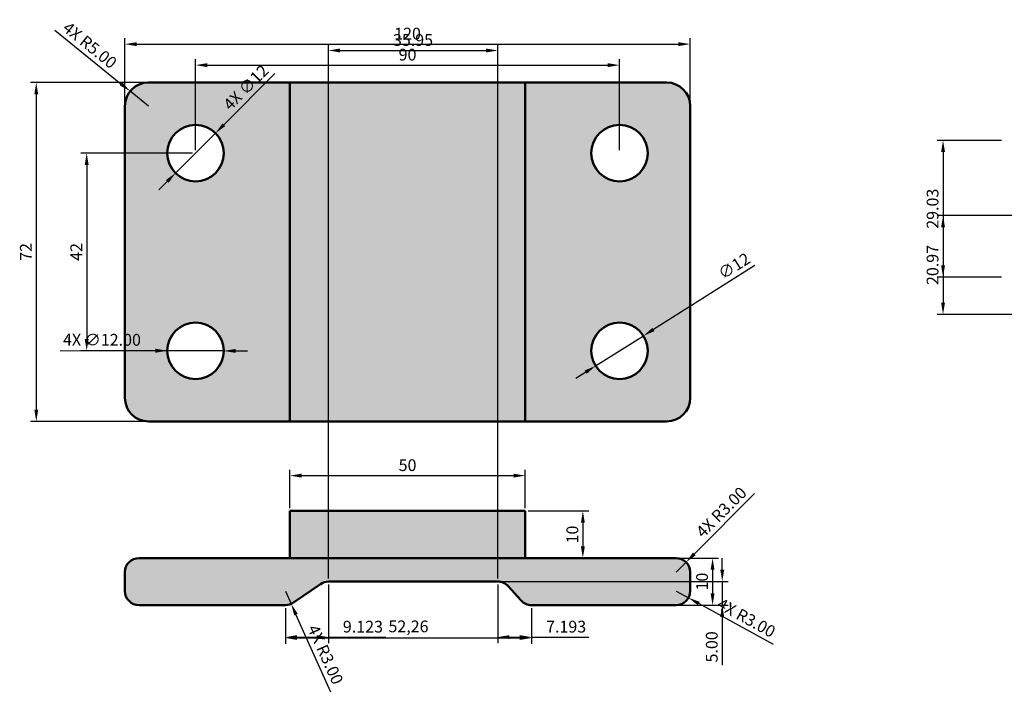
# Model space of a CAD drawing. Units: millimetres. Extents: x 1248 to 2192, y 1962 to 2325.
# Tile 2 of 4: x 1248 to 1457, y 2091 to 2234. Entities that reach past the tile are written whole.
import ezdxf

# ---------------------------------------------------------------- set-up
doc = ezdxf.new("R2010")
doc.units = ezdxf.units.MM
for name, color, linetype, lineweight in [('M-DIMS', 2, 'Continuous', 25), ('M-HATC', 8, 'Continuous', 18), ('M-OUTL', 7, 'Continuous', 50)]:
    doc.layers.add(name, color=color, linetype=linetype, lineweight=lineweight)
doc.styles.get("Standard").update_dxf_attribs({"font": 'arial.ttf'})
doc.dimstyles.new('ISO-25', dxfattribs={"dimtxt": 2.5, "dimasz": 2.5, "dimexe": 1.25, "dimexo": 0.625, "dimtad": 1, "dimtxsty": 'Standard', "dimcen": 2.5, "dimadec": 0, "dimazin": 0, "dimtfac": 1, "dimtmove": 0, "dimatfit": 3, "dimfxl": 1, "dimarcsym": 0})

# ---------------------------------------------------------------- blocks, each defined once
blk = doc.blocks.new('*D1')
at = {"layer": 'Defpoints', "color": 0, "transparency": 16777216}
for p in [(1285.59, 2205.19), (1262.48, 2163.19), (1285.59, 2163.19)]:
    blk.add_point(p, dxfattribs=at)
at = {"layer": 'M-DIMS', "color": 0, "lineweight": -2, "transparency": 16777216}
for p, q in [((1284.97, 2205.19), (1261.23, 2205.19)), ((1262.48, 2202.69), (1262.48, 2165.69)), ((1284.97, 2163.19), (1261.23, 2163.19))]:
    blk.add_line(p, q, dxfattribs=at)
at = {"layer": 'M-DIMS', "color": 0, "transparency": 16777216}
for points in [[(1262.07, 2202.69), (1262.9, 2202.69), (1262.48, 2205.19)], [(1262.07, 2165.69), (1262.9, 2165.69), (1262.48, 2163.19)]]:
    blk.add_solid(points, dxfattribs=at)
at = {"layer": 'M-DIMS', "color": 0, "transparency": 16777216, "insert": (1260.6, 2184.19), "char_height": 2.5, "attachment_point": 5, "rotation": 90}
blk.add_mtext('42', dxfattribs=at)
blk = doc.blocks.new('*D2')
at = {"layer": 'Defpoints', "color": 0, "transparency": 16777216}
for p in [(1275.59, 2220.19), (1251.78, 2148.19), (1275.59, 2148.19)]:
    blk.add_point(p, dxfattribs=at)
at = {"layer": 'M-DIMS', "color": 0, "lineweight": -2, "transparency": 16777216}
for p, q in [((1274.97, 2220.19), (1250.53, 2220.19)), ((1251.78, 2217.69), (1251.78, 2150.69)), ((1274.97, 2148.19), (1250.53, 2148.19))]:
    blk.add_line(p, q, dxfattribs=at)
at = {"layer": 'M-DIMS', "color": 0, "transparency": 16777216}
for points in [[(1251.37, 2217.69), (1252.2, 2217.69), (1251.78, 2220.19)], [(1251.37, 2150.69), (1252.2, 2150.69), (1251.78, 2148.19)]]:
    blk.add_solid(points, dxfattribs=at)
at = {"layer": 'M-DIMS', "color": 0, "transparency": 16777216, "insert": (1249.9, 2184.19), "char_height": 2.5, "attachment_point": 5, "rotation": 90}
blk.add_mtext('72', dxfattribs=at)
blk = doc.blocks.new('*D3')
at = {"layer": 'Defpoints', "color": 0, "transparency": 16777216}
for p in [(1390.59, 2228.33), (1270.59, 2215.19), (1390.59, 2215.19)]:
    blk.add_point(p, dxfattribs=at)
at = {"layer": 'M-DIMS', "color": 0, "lineweight": -2, "transparency": 16777216}
for p, q in [((1270.59, 2215.81), (1270.59, 2229.58)), ((1273.09, 2228.33), (1388.09, 2228.33)), ((1390.59, 2215.81), (1390.59, 2229.58))]:
    blk.add_line(p, q, dxfattribs=at)
at = {"layer": 'M-DIMS', "color": 0, "transparency": 16777216}
for points in [[(1273.09, 2228.75), (1273.09, 2227.92), (1270.59, 2228.33)], [(1388.09, 2228.75), (1388.09, 2227.92), (1390.59, 2228.33)]]:
    blk.add_solid(points, dxfattribs=at)
at = {"layer": 'M-DIMS', "color": 0, "transparency": 16777216, "insert": (1330.59, 2230.24), "char_height": 2.5, "attachment_point": 5}
blk.add_mtext('120', dxfattribs=at)
blk = doc.blocks.new('*D4')
at = {"layer": 'Defpoints', "color": 0, "transparency": 16777216}
for p in [(1375.59, 2223.87), (1285.59, 2205.19), (1375.59, 2205.19)]:
    blk.add_point(p, dxfattribs=at)
at = {"layer": 'M-DIMS', "color": 0, "lineweight": -2, "transparency": 16777216}
for p, q in [((1285.59, 2205.81), (1285.59, 2225.12)), ((1288.09, 2223.87), (1373.09, 2223.87)), ((1375.59, 2205.81), (1375.59, 2225.12))]:
    blk.add_line(p, q, dxfattribs=at)
at = {"layer": 'M-DIMS', "color": 0, "transparency": 16777216}
for points in [[(1288.09, 2224.29), (1288.09, 2223.46), (1285.59, 2223.87)], [(1373.09, 2224.29), (1373.09, 2223.46), (1375.59, 2223.87)]]:
    blk.add_solid(points, dxfattribs=at)
at = {"layer": 'M-DIMS', "color": 0, "transparency": 16777216, "insert": (1330.59, 2225.78), "char_height": 2.5, "attachment_point": 5}
blk.add_mtext('90', dxfattribs=at)
blk = doc.blocks.new('*D5')
at = {"layer": 'Defpoints', "color": 0, "transparency": 16777216}
for p in [(1380.67, 2166.38), (1370.52, 2159.99)]:
    blk.add_point(p, dxfattribs=at)
at = {"layer": 'M-DIMS', "color": 0, "lineweight": -2, "transparency": 16777216}
for p, q in [((1404.33, 2181.28), (1382.78, 2167.71)), ((1370.52, 2159.99), (1380.67, 2166.38)), ((1368.4, 2158.66), (1366.28, 2157.32))]:
    blk.add_line(p, q, dxfattribs=at)
at = {"layer": 'M-DIMS', "color": 0, "transparency": 16777216}
for points in [[(1382.56, 2168.07), (1383.01, 2167.36), (1380.67, 2166.38)], [(1368.18, 2159.01), (1368.62, 2158.3), (1370.52, 2159.99)]]:
    blk.add_solid(points, dxfattribs=at)
at = {"layer": 'M-DIMS', "color": 0, "transparency": 16777216, "insert": (1400.09, 2180.94), "char_height": 2.5, "attachment_point": 5, "rotation": 32.2006}
blk.add_mtext('∅12', dxfattribs=at)
blk = doc.blocks.new('*D6')
at = {"layer": 'Defpoints', "color": 0, "transparency": 16777216}
for p in [(1304.66, 2109.16), (1356.92, 2109.16), (1356.92, 2102.19)]:
    blk.add_point(p, dxfattribs=at)
at = {"layer": 'M-DIMS', "color": 0, "lineweight": -2, "transparency": 16777216}
for p, q in [((1304.66, 2108.54), (1304.66, 2100.94)), ((1356.92, 2108.54), (1356.92, 2100.94)), ((1307.16, 2102.19), (1354.42, 2102.19))]:
    blk.add_line(p, q, dxfattribs=at)
at = {"layer": 'M-DIMS', "color": 0, "transparency": 16777216}
for points in [[(1307.16, 2102.61), (1307.16, 2101.77), (1304.66, 2102.19)], [(1354.42, 2102.61), (1354.42, 2101.77), (1356.92, 2102.19)]]:
    blk.add_solid(points, dxfattribs=at)
at = {"layer": 'M-DIMS', "color": 0, "transparency": 16777216, "insert": (1330.79, 2104.32), "char_height": 2.5, "attachment_point": 5}
blk.add_mtext('52,26', dxfattribs=at)
blk = doc.blocks.new('*D7')
at = {"layer": 'Defpoints', "color": 0, "transparency": 16777216}
for p in [(1355.59, 2136.67), (1305.59, 2129.16), (1355.59, 2129.16)]:
    blk.add_point(p, dxfattribs=at)
at = {"layer": 'M-DIMS', "color": 0, "lineweight": -2, "transparency": 16777216}
for p, q in [((1305.59, 2129.79), (1305.59, 2137.92)), ((1308.09, 2136.67), (1353.09, 2136.67)), ((1355.59, 2129.79), (1355.59, 2137.92))]:
    blk.add_line(p, q, dxfattribs=at)
at = {"layer": 'M-DIMS', "color": 0, "transparency": 16777216}
for points in [[(1308.09, 2137.08), (1308.09, 2136.25), (1305.59, 2136.67)], [(1353.09, 2137.08), (1353.09, 2136.25), (1355.59, 2136.67)]]:
    blk.add_solid(points, dxfattribs=at)
at = {"layer": 'M-DIMS', "color": 0, "transparency": 16777216, "insert": (1330.59, 2138.57), "char_height": 2.5, "attachment_point": 5}
blk.add_mtext('50', dxfattribs=at)
blk = doc.blocks.new('*D8')
at = {"layer": 'Defpoints', "color": 0, "transparency": 16777216}
for p in [(1355.59, 2129.16), (1355.59, 2119.16), (1367.8, 2119.16)]:
    blk.add_point(p, dxfattribs=at)
at = {"layer": 'M-DIMS', "color": 0, "lineweight": -2, "transparency": 16777216}
for p, q in [((1356.22, 2129.16), (1369.05, 2129.16)), ((1367.8, 2126.66), (1367.8, 2121.66)), ((1356.22, 2119.16), (1369.05, 2119.16))]:
    blk.add_line(p, q, dxfattribs=at)
at = {"layer": 'M-DIMS', "color": 0, "transparency": 16777216}
for points in [[(1367.39, 2126.66), (1368.22, 2126.66), (1367.8, 2129.16)], [(1367.39, 2121.66), (1368.22, 2121.66), (1367.8, 2119.16)]]:
    blk.add_solid(points, dxfattribs=at)
at = {"layer": 'M-DIMS', "color": 0, "transparency": 16777216, "insert": (1365.9, 2124.16), "char_height": 2.5, "attachment_point": 5, "rotation": 90}
blk.add_mtext('10', dxfattribs=at)
blk = doc.blocks.new('*D9')
at = {"layer": 'Defpoints', "color": 0, "transparency": 16777216}
for p in [(1387.59, 2119.16), (1387.59, 2109.16), (1395.34, 2109.16)]:
    blk.add_point(p, dxfattribs=at)
at = {"layer": 'M-DIMS', "color": 0, "lineweight": -2, "transparency": 16777216}
for p, q in [((1388.22, 2119.16), (1396.59, 2119.16)), ((1395.34, 2116.66), (1395.34, 2111.66)), ((1388.22, 2109.16), (1396.59, 2109.16))]:
    blk.add_line(p, q, dxfattribs=at)
at = {"layer": 'M-DIMS', "color": 0, "transparency": 16777216}
for points in [[(1394.92, 2116.66), (1395.75, 2116.66), (1395.34, 2119.16)], [(1394.92, 2111.66), (1395.75, 2111.66), (1395.34, 2109.16)]]:
    blk.add_solid(points, dxfattribs=at)
at = {"layer": 'M-DIMS', "color": 0, "transparency": 16777216, "insert": (1393.43, 2114.16), "char_height": 2.5, "attachment_point": 5, "rotation": 90}
blk.add_mtext('10', dxfattribs=at)
blk = doc.blocks.new('*D39')
at = {"layer": 'Defpoints', "color": 0, "transparency": 16777216}
for p in [(1457.26, 2207.89), (1444.26, 2178.86), (1457.26, 2178.86)]:
    blk.add_point(p, dxfattribs=at)
at = {"layer": 'M-DIMS', "color": 0, "lineweight": -2, "transparency": 16777216}
for p, q in [((1456.64, 2207.89), (1443.01, 2207.89)), ((1444.26, 2205.39), (1444.26, 2181.36)), ((1456.64, 2178.86), (1443.01, 2178.86))]:
    blk.add_line(p, q, dxfattribs=at)
at = {"layer": 'M-DIMS', "color": 0, "transparency": 16777216}
for points in [[(1443.84, 2205.39), (1444.68, 2205.39), (1444.26, 2207.89)], [(1443.84, 2181.36), (1444.68, 2181.36), (1444.26, 2178.86)]]:
    blk.add_solid(points, dxfattribs=at)
at = {"layer": 'M-DIMS', "color": 0, "transparency": 16777216, "insert": (1442.36, 2193.37), "char_height": 2.5, "attachment_point": 5, "rotation": 90}
blk.add_mtext('29.03', dxfattribs=at)
blk = doc.blocks.new('*D40')
at = {"layer": 'Defpoints', "color": 0, "transparency": 16777216}
for p in [(1571.8, 2191.9), (1444.26, 2170.93), (1498.95, 2170.93)]:
    blk.add_point(p, dxfattribs=at)
at = {"layer": 'M-DIMS', "color": 0, "lineweight": -2, "transparency": 16777216}
for p, q in [((1571.17, 2191.9), (1443.01, 2191.9)), ((1444.26, 2189.4), (1444.26, 2173.43)), ((1498.32, 2170.93), (1443.01, 2170.93))]:
    blk.add_line(p, q, dxfattribs=at)
at = {"layer": 'M-DIMS', "color": 0, "transparency": 16777216}
for points in [[(1443.84, 2189.4), (1444.68, 2189.4), (1444.26, 2191.9)], [(1443.84, 2173.43), (1444.68, 2173.43), (1444.26, 2170.93)]]:
    blk.add_solid(points, dxfattribs=at)
at = {"layer": 'M-DIMS', "color": 0, "transparency": 16777216, "insert": (1442.36, 2181.42), "char_height": 2.5, "attachment_point": 5, "rotation": 90}
blk.add_mtext('20.97', dxfattribs=at)
blk = doc.blocks.new('*D56')
at = {"layer": 'Defpoints', "color": 0, "transparency": 16777216}
for p in [(1289.83, 2209.43), (1281.35, 2200.94)]:
    blk.add_point(p, dxfattribs=at)
at = {"layer": 'M-DIMS', "color": 0, "lineweight": -2, "transparency": 16777216}
for p, q in [((1302.45, 2222.07), (1291.6, 2211.2)), ((1281.35, 2200.94), (1289.83, 2209.43)), ((1279.59, 2199.17), (1277.82, 2197.4))]:
    blk.add_line(p, q, dxfattribs=at)
at = {"layer": 'M-DIMS', "color": 0, "transparency": 16777216}
for points in [[(1291.3, 2211.5), (1291.89, 2210.91), (1289.83, 2209.43)], [(1279.29, 2199.46), (1279.88, 2198.88), (1281.35, 2200.94)]]:
    blk.add_solid(points, dxfattribs=at)
at = {"layer": 'M-DIMS', "color": 0, "transparency": 16777216, "insert": (1296.51, 2218.91), "char_height": 2.5, "attachment_point": 5, "rotation": 45.0476}
blk.add_mtext('4X ∅12', dxfattribs=at)
blk = doc.blocks.new('*D65')
at = {"layer": 'Defpoints', "color": 0, "transparency": 16777216}
for p in [(1349.73, 2226.99), (1313.78, 2114.16), (1349.73, 2114.16)]:
    blk.add_point(p, dxfattribs=at)
at = {"layer": 'M-DIMS', "color": 0, "lineweight": -2, "transparency": 16777216}
for p, q in [((1313.78, 2114.79), (1313.78, 2228.24)), ((1349.73, 2114.79), (1349.73, 2228.24)), ((1316.28, 2226.99), (1347.23, 2226.99))]:
    blk.add_line(p, q, dxfattribs=at)
at = {"layer": 'M-DIMS', "color": 0, "transparency": 16777216}
for points in [[(1316.28, 2227.4), (1316.28, 2226.57), (1313.78, 2226.99)], [(1347.23, 2227.4), (1347.23, 2226.57), (1349.73, 2226.99)]]:
    blk.add_solid(points, dxfattribs=at)
at = {"layer": 'M-DIMS', "color": 0, "transparency": 16777216, "insert": (1331.75, 2228.89), "char_height": 2.5, "attachment_point": 5}
blk.add_mtext('35.95', dxfattribs=at)
blk = doc.blocks.new('*D66')
at = {"layer": 'Defpoints', "color": 0, "transparency": 16777216}
for p in [(1349.73, 2114.16), (1356.92, 2109.16), (1397.39, 2109.16)]:
    blk.add_point(p, dxfattribs=at)
at = {"layer": 'M-DIMS', "color": 0, "lineweight": -2, "transparency": 16777216}
for p, q in [((1397.39, 2116.66), (1397.39, 2119.16)), ((1350.35, 2114.16), (1398.64, 2114.16)), ((1397.39, 2114.16), (1397.39, 2109.16)), ((1357.55, 2109.16), (1398.64, 2109.16)), ((1397.39, 2106.66), (1397.39, 2096.43))]:
    blk.add_line(p, q, dxfattribs=at)
at = {"layer": 'M-DIMS', "color": 0, "transparency": 16777216}
for points in [[(1396.98, 2116.66), (1397.81, 2116.66), (1397.39, 2114.16)], [(1396.98, 2106.66), (1397.81, 2106.66), (1397.39, 2109.16)]]:
    blk.add_solid(points, dxfattribs=at)
at = {"layer": 'M-DIMS', "color": 0, "transparency": 16777216, "insert": (1395.49, 2100.29), "char_height": 2.5, "attachment_point": 5, "rotation": 90}
blk.add_mtext('5.00', dxfattribs=at)
blk = doc.blocks.new('*D67')
at = {"layer": 'Defpoints', "color": 0, "transparency": 16777216}
for p in [(1313.78, 2114.16), (1304.66, 2109.16), (1313.78, 2102.36)]:
    blk.add_point(p, dxfattribs=at)
at = {"layer": 'M-DIMS', "color": 0, "lineweight": -2, "transparency": 16777216}
for p, q in [((1313.78, 2113.54), (1313.78, 2101.11)), ((1304.66, 2108.54), (1304.66, 2101.11)), ((1307.16, 2102.36), (1311.28, 2102.36)), ((1313.78, 2102.36), (1325.97, 2102.36))]:
    blk.add_line(p, q, dxfattribs=at)
at = {"layer": 'M-DIMS', "color": 0, "transparency": 16777216}
for points in [[(1307.16, 2102.78), (1307.16, 2101.94), (1304.66, 2102.36)], [(1311.28, 2102.78), (1311.28, 2101.94), (1313.78, 2102.36)]]:
    blk.add_solid(points, dxfattribs=at)
at = {"layer": 'M-DIMS', "color": 0, "transparency": 16777216, "insert": (1321.12, 2104.26), "char_height": 2.5, "attachment_point": 5}
blk.add_mtext('9.123', dxfattribs=at)
blk = doc.blocks.new('*D68')
at = {"layer": 'Defpoints', "color": 0, "transparency": 16777216}
for p in [(1349.73, 2114.16), (1356.92, 2109.16), (1356.92, 2102.36)]:
    blk.add_point(p, dxfattribs=at)
at = {"layer": 'M-DIMS', "color": 0, "lineweight": -2, "transparency": 16777216}
for p, q in [((1349.73, 2113.54), (1349.73, 2101.11)), ((1356.92, 2108.54), (1356.92, 2101.11)), ((1352.23, 2102.36), (1354.42, 2102.36)), ((1356.92, 2102.36), (1369.09, 2102.36))]:
    blk.add_line(p, q, dxfattribs=at)
at = {"layer": 'M-DIMS', "color": 0, "transparency": 16777216}
for points in [[(1352.23, 2102.78), (1352.23, 2101.94), (1349.73, 2102.36)], [(1354.42, 2102.78), (1354.42, 2101.94), (1356.92, 2102.36)]]:
    blk.add_solid(points, dxfattribs=at)
at = {"layer": 'M-DIMS', "color": 0, "transparency": 16777216, "insert": (1364.25, 2104.26), "char_height": 2.5, "attachment_point": 5}
blk.add_mtext('7.193', dxfattribs=at)
blk = doc.blocks.new('*D75')
at = {"layer": 'Defpoints', "color": 0, "transparency": 16777216}
for p in [(1279.59, 2163.2), (1291.59, 2163.17)]:
    blk.add_point(p, dxfattribs=at)
at = {"layer": 'M-DIMS', "color": 0, "lineweight": -2, "transparency": 16777216}
for p, q in [((1256.86, 2163.26), (1277.09, 2163.21)), ((1291.59, 2163.17), (1279.59, 2163.2)), ((1294.09, 2163.16), (1296.59, 2163.16))]:
    blk.add_line(p, q, dxfattribs=at)
at = {"layer": 'M-DIMS', "color": 0, "transparency": 16777216}
for points in [[(1277.09, 2163.62), (1277.09, 2162.79), (1279.59, 2163.2)], [(1294.09, 2163.58), (1294.09, 2162.75), (1291.59, 2163.17)]]:
    blk.add_solid(points, dxfattribs=at)
at = {"layer": 'M-DIMS', "color": 0, "transparency": 16777216, "insert": (1265.73, 2165.21), "char_height": 2.5, "attachment_point": 5, "rotation": 359.8595}
blk.add_mtext('4X ∅12.00', dxfattribs=at)
blk = doc.blocks.new('*D78')
at = {"layer": 'Defpoints', "color": 0, "transparency": 16777216}
for p in [(1271.71, 2218.33), (1275.59, 2215.19)]:
    blk.add_point(p, dxfattribs=at)
at = {"layer": 'M-DIMS', "color": 0, "lineweight": -2, "transparency": 16777216}
for p, q in [((1255.7, 2231.3), (1269.76, 2219.91)), ((1275.59, 2215.19), (1271.71, 2218.33))]:
    blk.add_line(p, q, dxfattribs=at)
at = {"layer": 'M-DIMS', "color": 0, "transparency": 16777216}
blk.add_solid([(1270.03, 2220.23), (1269.5, 2219.58), (1271.71, 2218.33)], dxfattribs=at)
at = {"layer": 'M-DIMS', "color": 0, "transparency": 16777216, "insert": (1262.96, 2227.87), "char_height": 2.5, "attachment_point": 5, "rotation": 320.9935}
blk.add_mtext('4X R5.00', dxfattribs=at)
blk = doc.blocks.new('*D79')
at = {"layer": 'Defpoints', "color": 0, "transparency": 16777216}
for p in [(1387.59, 2112.16), (1390.22, 2110.71)]:
    blk.add_point(p, dxfattribs=at)
at = {"layer": 'M-DIMS', "color": 0, "lineweight": -2, "transparency": 16777216}
for p, q in [((1387.59, 2112.16), (1390.22, 2110.71)), ((1408.26, 2100.78), (1392.41, 2109.51))]:
    blk.add_line(p, q, dxfattribs=at)
at = {"layer": 'M-DIMS', "color": 0, "transparency": 16777216}
blk.add_solid([(1392.61, 2109.87), (1392.21, 2109.14), (1390.22, 2110.71)], dxfattribs=at)
at = {"layer": 'M-DIMS', "color": 0, "transparency": 16777216, "insert": (1402.35, 2106.2), "char_height": 2.5, "attachment_point": 5, "rotation": 331.1567}
blk.add_mtext('4X R3.00', dxfattribs=at)
blk = doc.blocks.new('*D80')
at = {"layer": 'Defpoints', "color": 0, "transparency": 16777216}
for p in [(1304.66, 2112.16), (1305.89, 2109.42)]:
    blk.add_point(p, dxfattribs=at)
at = {"layer": 'M-DIMS', "color": 0, "lineweight": -2, "transparency": 16777216}
for p, q in [((1304.66, 2112.16), (1305.89, 2109.42)), ((1314.34, 2090.64), (1306.91, 2107.14))]:
    blk.add_line(p, q, dxfattribs=at)
at = {"layer": 'M-DIMS', "color": 0, "transparency": 16777216}
blk.add_solid([(1307.29, 2107.32), (1306.53, 2106.97), (1305.89, 2109.42)], dxfattribs=at)
at = {"layer": 'M-DIMS', "color": 0, "transparency": 16777216, "insert": (1312.87, 2098.53), "char_height": 2.5, "attachment_point": 5, "rotation": 294.2089}
blk.add_mtext('4X R3.00', dxfattribs=at)
blk = doc.blocks.new('*D81')
at = {"layer": 'Defpoints', "color": 0, "transparency": 16777216}
for p in [(1389.71, 2118.28), (1387.59, 2116.16)]:
    blk.add_point(p, dxfattribs=at)
at = {"layer": 'M-DIMS', "color": 0, "lineweight": -2, "transparency": 16777216}
for p, q in [((1404.27, 2132.85), (1391.48, 2120.05)), ((1387.59, 2116.16), (1389.71, 2118.28))]:
    blk.add_line(p, q, dxfattribs=at)
at = {"layer": 'M-DIMS', "color": 0, "transparency": 16777216}
blk.add_solid([(1391.19, 2120.35), (1391.77, 2119.76), (1389.71, 2118.28)], dxfattribs=at)
at = {"layer": 'M-DIMS', "color": 0, "transparency": 16777216, "insert": (1397.41, 2128.68), "char_height": 2.5, "attachment_point": 5, "rotation": 45.0215}
blk.add_mtext('4X R3.00', dxfattribs=at)

msp = doc.modelspace()

# ---------------------------------------------------------------- hatches: boundary and pattern name
at = {"layer": 'M-HATC'}
h = msp.add_hatch(color=256, dxfattribs=at)
h.set_gradient(color1=(147, 39, 143), color2=(147, 39, 143))
h.paths.add_polyline_path([(1270.5924, 2153.1853, 0.41421356), (1275.5924, 2148.1853), (1305.5924, 2148.1853), (1305.5924, 2220.1853), (1275.5924, 2220.1853, 0.41421356), (1270.5924, 2215.1853)])
h.paths.add_polyline_path([(1279.5924, 2205.1853, -1), (1291.5924, 2205.1853, -1)], flags=16)
h.paths.add_polyline_path([(1291.5924, 2163.1853, -1), (1279.5924, 2163.1853, -1)], flags=16)
h.paths.add_polyline_path([(1305.5924, 2148.1853), (1330.5924, 2148.1853), (1355.5924, 2148.1853), (1355.5924, 2220.1853), (1305.5924, 2220.1853)])
h.paths.add_polyline_path([(1390.5924, 2215.1853, 0.41421356), (1385.5924, 2220.1853), (1355.5924, 2220.1853), (1355.5924, 2148.1853), (1385.5924, 2148.1853, 0.41421356), (1390.5924, 2153.1853)])
h.paths.add_polyline_path([(1369.5924, 2205.1853, -1), (1381.5924, 2205.1853, -1)], flags=16)
h.paths.add_polyline_path([(1381.5924, 2163.1853, -1), (1369.5924, 2163.1853, -1)], flags=16)
h = msp.add_hatch(color=256, dxfattribs=at)
h.set_gradient(color1=(100, 33, 101), color2=(100, 33, 101))
h.paths.add_polyline_path([(1313.7813, 2114.1608), (1349.7285, 2114.1608, -0.21162092), (1351.9508, 2113.1761), (1354.6994, 2110.1454, 0.21162092), (1356.9216, 2109.1608), (1387.5924, 2109.1608, 0.41421356), (1390.5924, 2112.1608), (1390.5924, 2116.1608, 0.41421356), (1387.5924, 2119.1608), (1273.5924, 2119.1608, 0.41421356), (1270.5924, 2116.1608), (1270.5924, 2112.1608, 0.41421356), (1273.5924, 2109.1608), (1304.6587, 2109.1608, 0.15200558), (1306.3611, 2109.6905), (1312.079, 2113.631, -0.15200558)])
h.paths.add_polyline_path([(1355.5924, 2129.1608), (1305.5924, 2129.1608), (1305.5924, 2119.1608), (1355.5924, 2119.1608)])

# ---------------------------------------------------------------- linework, layer by layer
at = {"layer": 'M-OUTL'}
for p, q in [((1275.5924, 2220.1853), (1385.5924, 2220.1853)), ((1305.5924, 2148.1853), (1305.5924, 2220.1853)), ((1355.5924, 2220.1853), (1355.5924, 2148.1853)), ((1270.5924, 2153.1853), (1270.5924, 2215.1853)), ((1390.5924, 2215.1853), (1390.5924, 2153.1853)), ((1385.5924, 2148.1853), (1275.5924, 2148.1853)), ((1330.5924, 2148.1853), (1305.5924, 2148.1853)), ((1305.5924, 2119.1608), (1305.5924, 2129.1608)), ((1305.5924, 2129.1608), (1355.5924, 2129.1608)), ((1355.5924, 2129.1608), (1355.5924, 2119.1608)), ((1273.5924, 2119.1608), (1387.5924, 2119.1608)), ((1270.5924, 2116.1608), (1270.5924, 2112.1608)), ((1390.5924, 2112.1608), (1390.5924, 2116.1608)), ((1306.3611, 2109.6905), (1312.079, 2113.631)), ((1313.7813, 2114.1608), (1349.7285, 2114.1608)), ((1354.6994, 2110.1454), (1351.9508, 2113.1761)), ((1273.5924, 2109.1608), (1304.6587, 2109.1608)), ((1356.9216, 2109.1608), (1387.5924, 2109.1608))]:
    msp.add_line(p, q, dxfattribs=at)
for centre in [(1285.5924, 2205.1853), (1375.5924, 2205.1853), (1285.5924, 2163.1853), (1375.5924, 2163.1853)]:
    msp.add_circle(centre, 6, dxfattribs=at)
for centre, radius, start, end in [((1275.5924, 2215.1853), 5, 90, 180), ((1385.5924, 2215.1853), 5, 0, 90), ((1275.5924, 2153.1853), 5, 180, 270), ((1385.5924, 2153.1853), 5, 270, 0), ((1273.5924, 2116.1608), 3, 90, 180), ((1387.5924, 2116.1608), 3, 0, 90), ((1313.7813, 2111.1608), 3, 90, 124.57246), ((1349.7285, 2111.1608), 3, 42.205204, 90), ((1273.5924, 2112.1608), 3, 180, 270), ((1387.5924, 2112.1608), 3, 270, 0), ((1304.6587, 2112.1608), 3, 270, 304.57246), ((1356.9216, 2112.1608), 3, 222.205204, 270)]:
    msp.add_arc(centre, radius, start, end, dxfattribs=at)

# ---------------------------------------------------------------- dimensions: what is measured, and where the dimension line sits
at = {"layer": 'M-DIMS'}
for center, mpoint, picture, middle in [((1275.5924, 2215.1853), (1271.707, 2218.3324), '*D78', (1262.9571, 2227.8664)), ((1387.5924, 2116.1608), (1389.7129, 2118.2829), '*D81', (1397.4149, 2128.682)), ((1304.6587, 2112.1608), (1305.8889, 2109.4246), '*D80', (1312.8728, 2098.5302)), ((1387.5924, 2112.1608), (1390.2202, 2110.7135), '*D79', (1402.3501, 2106.2048))]:
    dim = msp.add_radius_dim(center=center, mpoint=mpoint, text='4X <>', dimstyle='ISO-25', override={"dimdec": 2, "dimlfac": 1, "dimrnd": 0, "dimzin": 0, "dimdsep": 46, "dimlunit": 2}, dxfattribs=at)
    dim.commit()
    dim.dimension.update_dxf_attribs({"geometry": picture, "text_midpoint": middle})
for base, p1, p2, override, picture, middle in [((1390.5924, 2228.3349), (1270.5924, 2215.1853), (1390.5924, 2215.1853), {"dimclrd": 0, "dimclre": 0, "dimclrt": 0}, '*D3', (1330.5924, 2230.2363)), ((1349.7285, 2226.9853), (1313.7813, 2114.1608), (1349.7285, 2114.1608), {"dimdec": 2, "dimlfac": 1, "dimrnd": 0, "dimzin": 0, "dimdsep": 46, "dimlunit": 2}, '*D65', (1331.7549, 2228.8876)), ((1375.5924, 2223.874), (1285.5924, 2205.1853), (1375.5924, 2205.1853), {"dimclrd": 0, "dimclre": 0, "dimclrt": 0}, '*D4', (1330.5924, 2225.7754)), ((1355.5924, 2136.6679), (1305.5924, 2129.1608), (1355.5924, 2129.1608), {"dimclrd": 0, "dimclre": 0, "dimclrt": 0}, '*D7', (1330.5924, 2138.5693)), ((1313.7813, 2102.3608), (1304.6587, 2109.1608), (1313.7813, 2114.1608), {"dimdec": 3, "dimlfac": 1, "dimrnd": 0, "dimzin": 0, "dimdsep": 46, "dimlunit": 2}, '*D67', (1321.1244, 2104.263)), ((1356.9216, 2102.3608), (1349.7285, 2114.1608), (1356.9216, 2109.1608), {"dimdec": 3, "dimlfac": 1, "dimrnd": 0, "dimzin": 0, "dimdsep": 46, "dimlunit": 2}, '*D68', (1364.2545, 2104.263)), ((1356.9216, 2102.1903), (1304.6587, 2109.1608), (1356.9216, 2109.1608), {"dimclrd": 0, "dimclre": 0, "dimclrt": 0}, '*D6', (1330.7902, 2104.3177))]:
    dim = msp.add_linear_dim(base=base, p1=p1, p2=p2, dimstyle='ISO-25', override=override, dxfattribs=at)
    dim.commit()
    dim.dimension.update_dxf_attribs({"geometry": picture, "text_midpoint": middle})
dim = msp.add_diameter_dim_2p(p1=(1281.3532, 2200.9391), p2=(1289.8315, 2209.4315), text='4X <>', dimstyle='ISO-25', override={"dimdec": 0, "dimlfac": 1, "dimrnd": 0, "dimzin": 0, "dimdsep": 46, "dimlunit": 2}, dxfattribs=at)
dim.commit()
dim.dimension.update_dxf_attribs({"geometry": '*D56', "text_midpoint": (1297.9087, 2217.5222)})
for base, p1, p2, override, picture, middle in [((1251.7844, 2148.1853), (1275.5924, 2220.1853), (1275.5924, 2148.1853), {"dimclrd": 0, "dimclre": 0, "dimclrt": 0}, '*D2', (1249.9043, 2184.1853)), ((1444.2612, 2178.8583), (1457.2612, 2207.8886), (1457.2612, 2178.8583), {"dimdec": 2, "dimlfac": 1, "dimrnd": 0, "dimzin": 0, "dimdsep": 46, "dimlunit": 2}, '*D39', (1442.3589, 2193.3734)), ((1262.4832, 2163.1853), (1285.5924, 2205.1853), (1285.5924, 2163.1853), {"dimclrd": 0, "dimclre": 0, "dimclrt": 0}, '*D1', (1260.6031, 2184.1853)), ((1444.2612, 2170.9312), (1571.7998, 2191.9009), (1498.9499, 2170.9312), {"dimdec": 2, "dimlfac": 1, "dimrnd": 0, "dimzin": 0, "dimdsep": 46, "dimlunit": 2}, '*D40', (1442.3598, 2181.4161)), ((1367.8036, 2119.1608), (1355.5924, 2129.1608), (1355.5924, 2119.1608), {"dimclrd": 0, "dimclre": 0, "dimclrt": 0}, '*D8', (1365.9022, 2124.1608)), ((1397.3924, 2109.1608), (1349.7285, 2114.1608), (1356.9216, 2109.1608), {"dimdec": 2, "dimlfac": 1, "dimrnd": 0, "dimzin": 0, "dimdsep": 46, "dimlunit": 2}, '*D66', (1395.4909, 2100.2931)), ((1395.3355, 2109.1608), (1387.5924, 2119.1608), (1387.5924, 2109.1608), {"dimclrd": 0, "dimclre": 0, "dimclrt": 0}, '*D9', (1393.434, 2114.1608))]:
    dim = msp.add_linear_dim(base=base, p1=p1, p2=p2, angle=90, dimstyle='ISO-25', override=override, dxfattribs=at)
    dim.commit()
    dim.dimension.update_dxf_attribs({"geometry": picture, "text_midpoint": middle})
dim = msp.add_diameter_dim_2p(p1=(1370.5152, 2159.988), p2=(1380.6695, 2166.3826), dimstyle='ISO-25', override={"dimclrd": 0, "dimclre": 0, "dimclrt": 0}, dxfattribs=at)
dim.commit()
dim.dimension.update_dxf_attribs({"geometry": '*D5', "text_midpoint": (1401.1422, 2179.2753), "dimtype": 163})
dim = msp.add_diameter_dim_2p(p1=(1291.5923, 2163.1706), p2=(1279.5924, 2163.2), text='4X <>', dimstyle='ISO-25', override={"dimdec": 2, "dimlfac": 1, "dimrnd": 0, "dimzin": 0, "dimdsep": 46, "dimlunit": 2}, dxfattribs=at)
dim.commit()
dim.dimension.update_dxf_attribs({"geometry": '*D75', "text_midpoint": (1265.7239, 2163.234), "dimtype": 163})

doc.saveas('drawing.dxf')
